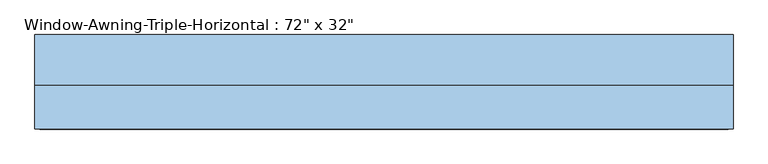
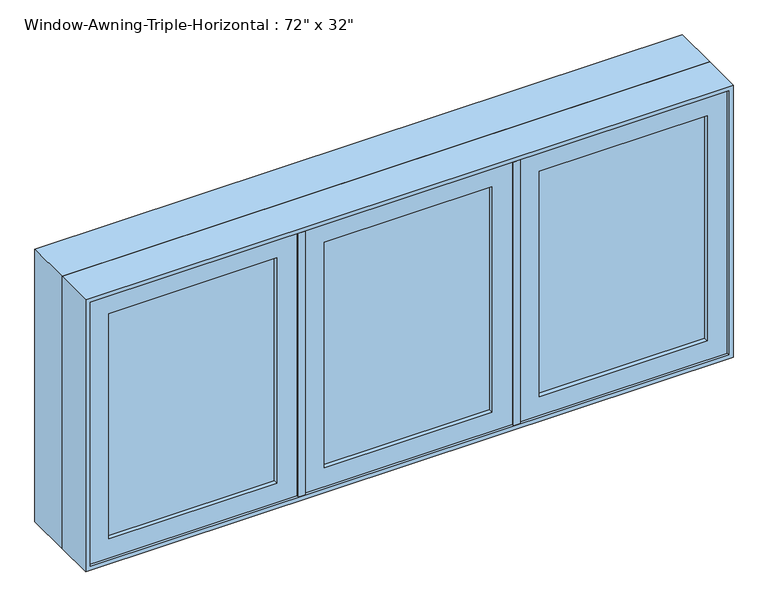
"""IFC4 building model written with IfcOpenShell, lengths in millimetres: window geometry."""

from ifc_helpers import new_model, si_unit, frame, origin, place, context, project, spatial, polyline, outline, extrude, faceted_brep, source, transform, mapped, element, save


def window_33d4544c(model_context):
    return source(origin(), model_context, "Body", "SolidModel", [
        faceted_brep([(882.65, -82.55, 1695.45), (-882.65, -82.55, 1695.45), (-882.65, -19.05, 1695.45), (882.65, -19.05, 1695.45), (901.7, -133.35, 1714.5), (-901.7, -133.35, 1714.5), (-901.7, -82.55, 1714.5), (901.7, -82.55, 1714.5), (914.4, -19.05, 1727.2), (-914.4, -19.05, 1727.2), (-914.4, -133.35, 1727.2), (914.4, -133.35, 1727.2), (-882.65, -82.55, 946.15), (-882.65, -19.05, 946.15), (-901.7, -133.35, 927.1), (-901.7, -82.55, 927.1), (-914.4, -19.05, 914.4), (-914.4, -133.35, 914.4), (882.65, -82.55, 946.15), (882.65, -19.05, 946.15), (901.7, -133.35, 927.1), (901.7, -82.55, 927.1), (914.4, -19.05, 914.4), (914.4, -133.35, 914.4)], [[[0, 1, 2, 3]], [[4, 5, 6, 7]], [[8, 9, 10, 11]], [[1, 12, 13, 2]], [[5, 14, 15, 6]], [[9, 16, 17, 10]], [[12, 18, 19, 13]], [[14, 20, 21, 15]], [[16, 22, 23, 17]], [[9, 8, 22, 16], [3, 2, 13, 19]], [[18, 0, 3, 19]], [[7, 6, 15, 21], [1, 0, 18, 12]], [[20, 4, 7, 21]], [[22, 8, 11, 23]], [[11, 10, 17, 23], [5, 4, 20, 14]]]),
        extrude(outline(polyline([(1727.2, -914.4), (914.4, -914.4), (914.4, 914.4), (1727.2, 914.4), (1727.2, -914.4)]), holes=[polyline([(1708.15, 895.35), (933.45, 895.35), (933.45, -895.35), (1708.15, -895.35), (1708.15, 895.35)])]), frame((0.0, -19.05, 0.0), z_axis=(0.0, 1.0, 0.0), x_axis=(0.0, 0.0, 1.0)), (0.0, 0.0, 1.0), 133.35),
        extrude(outline(polyline([(927.1, 313.2666667), (927.1, 901.7), (1714.5, 901.7), (1714.5, 313.2666667), (927.1, 313.2666667)]), holes=[polyline([(984.25, 844.55), (984.25, 370.4166667), (1657.35, 370.4166667), (1657.35, 844.55), (984.25, 844.55)])]), frame((0.0, -127.0, 0.0), z_axis=(0.0, 1.0, 0.0), x_axis=(0.0, 0.0, 1.0)), (0.0, 0.0, 1.0), 44.45),
        extrude(outline(polyline([(1714.5, -313.2666667), (1714.5, -901.7), (927.1, -901.7), (927.1, -313.2666667), (1714.5, -313.2666667)]), holes=[polyline([(1657.35, -844.55), (1657.35, -370.4166667), (984.25, -370.4166667), (984.25, -844.55), (1657.35, -844.55)])]), frame((0.0, -127.0, 0.0), z_axis=(0.0, 1.0, 0.0), x_axis=(0.0, 0.0, 1.0)), (0.0, 0.0, 1.0), 44.45),
        extrude(outline(polyline([(844.55, -114.3), (370.4166667, -114.3), (370.4166667, -107.95), (844.55, -107.95), (844.55, -114.3)])), frame((0.0, 0.0, 984.25), z_axis=(0.0, 0.0, 1.0), x_axis=(1.0, 0.0, 0.0)), (0.0, 0.0, 1.0), 673.1),
        extrude(outline(polyline([(370.4166667, -95.25), (844.55, -95.25), (844.55, -101.6), (370.4166667, -101.6), (370.4166667, -95.25)])), frame((0.0, 0.0, 984.25), z_axis=(0.0, 0.0, 1.0), x_axis=(1.0, 0.0, 0.0)), (0.0, 0.0, 1.0), 673.1),
        extrude(outline(polyline([(-370.4166667, -114.3), (-844.55, -114.3), (-844.55, -107.95), (-370.4166667, -107.95), (-370.4166667, -114.3)])), frame((0.0, 0.0, 984.25), z_axis=(0.0, 0.0, 1.0), x_axis=(1.0, 0.0, 0.0)), (0.0, 0.0, 1.0), 673.1),
        extrude(outline(polyline([(-844.55, -95.25), (-370.4166667, -95.25), (-370.4166667, -101.6), (-844.55, -101.6), (-844.55, -95.25)])), frame((0.0, 0.0, 984.25), z_axis=(0.0, 0.0, 1.0), x_axis=(1.0, 0.0, 0.0)), (0.0, 0.0, 1.0), 673.1),
        extrude(outline(polyline([(237.0666667, -114.3), (-237.0666667, -114.3), (-237.0666667, -107.95), (237.0666667, -107.95), (237.0666667, -114.3)])), frame((0.0, 0.0, 984.25), z_axis=(0.0, 0.0, 1.0), x_axis=(1.0, 0.0, 0.0)), (0.0, 0.0, 1.0), 673.1),
        extrude(outline(polyline([(-237.0666667, -95.25), (237.0666667, -95.25), (237.0666667, -101.6), (-237.0666667, -101.6), (-237.0666667, -95.25)])), frame((0.0, 0.0, 984.25), z_axis=(0.0, 0.0, 1.0), x_axis=(1.0, 0.0, 0.0)), (0.0, 0.0, 1.0), 673.1),
        extrude(outline(polyline([(927.1, -294.2166667), (927.1, 294.2166667), (1714.5, 294.2166667), (1714.5, -294.2166667), (927.1, -294.2166667)]), holes=[polyline([(984.25, 237.0666667), (984.25, -237.0666667), (1657.35, -237.0666667), (1657.35, 237.0666667), (984.25, 237.0666667)])]), frame((0.0, -127.0, 0.0), z_axis=(0.0, 1.0, 0.0), x_axis=(0.0, 0.0, 1.0)), (0.0, 0.0, 1.0), 44.45),
        faceted_brep([(294.2166667, -82.55, 1714.5), (294.2166667, -133.35, 1714.5), (313.2666667, -133.35, 1714.5), (313.2666667, -82.55, 1714.5), (333.7768005, -82.55, 1714.5), (333.7768005, -19.05, 1714.5), (273.7065328, -19.05, 1714.5), (273.7065328, -82.55, 1714.5), (294.2166667, -133.35, 927.1), (294.2166667, -104.775, 927.1), (313.2666667, -104.775, 927.1), (313.2666667, -133.35, 927.1), (273.7065328, -82.55, 1708.15), (294.2166667, -82.55, 1708.15), (294.2166667, -82.55, 1695.45), (273.7065328, -82.55, 1695.45), (273.7065328, -82.55, 946.15), (294.2166667, -82.55, 946.15), (273.7065328, -19.05, 1708.15), (273.7065328, -19.05, 1695.45), (273.7065328, -19.05, 946.15), (333.7768005, -19.05, 1708.15), (333.7768005, -19.05, 1695.45), (333.7768005, -19.05, 946.15), (333.7768005, -82.55, 1708.15), (333.7768005, -82.55, 1695.45), (333.7768005, -82.55, 946.15), (313.2666667, -82.55, 1708.15), (313.2666667, -82.55, 1695.45), (313.2666667, -82.55, 946.15), (313.2666667, -104.775, 946.15), (313.2666667, -104.775, 1695.45), (313.2666667, -104.775, 1708.15), (294.2166667, -104.775, 1708.15), (294.2166667, -104.775, 1695.45), (294.2166667, -104.775, 946.15)], [[[0, 1, 2, 3, 4, 5, 6, 7]], [[8, 9, 10, 11]], [[7, 12, 13, 0]], [[14, 15, 16, 17]], [[6, 18, 12, 7]], [[15, 19, 20, 16]], [[5, 21, 18, 6]], [[19, 22, 23, 20]], [[4, 24, 21, 5]], [[22, 25, 26, 23]], [[3, 27, 24, 4]], [[25, 28, 29, 26]], [[2, 11, 10, 30, 29, 28, 31, 32, 27, 3]], [[0, 13, 33, 34, 14, 17, 35, 9, 8, 1]], [[32, 31, 34, 33]], [[30, 10, 9, 35]], [[33, 13, 12, 18, 21, 24, 27, 32]], [[31, 28, 25, 22, 19, 15, 14, 34]], [[35, 17, 16, 20, 23, 26, 29, 30]], [[1, 8, 11, 2]]]),
        faceted_brep([(-313.2666667, -82.55, 1714.5), (-313.2666667, -133.35, 1714.5), (-294.2166667, -133.35, 1714.5), (-294.2166667, -82.55, 1714.5), (-273.7065328, -82.55, 1714.5), (-273.7065328, -19.05, 1714.5), (-333.7768005, -19.05, 1714.5), (-333.7768005, -82.55, 1714.5), (-313.2666667, -133.35, 927.1), (-313.2666667, -104.775, 927.1), (-294.2166667, -104.775, 927.1), (-294.2166667, -133.35, 927.1), (-333.7768005, -19.05, 1708.15), (-333.7768005, -82.55, 1708.15), (-333.7768005, -82.55, 1695.45), (-333.7768005, -19.05, 1695.45), (-333.7768005, -19.05, 946.15), (-333.7768005, -82.55, 946.15), (-273.7065328, -19.05, 1708.15), (-273.7065328, -19.05, 1695.45), (-273.7065328, -19.05, 946.15), (-273.7065328, -82.55, 1708.15), (-273.7065328, -82.55, 1695.45), (-273.7065328, -82.55, 946.15), (-294.2166667, -104.775, 946.15), (-294.2166667, -82.55, 946.15), (-294.2166667, -82.55, 1695.45), (-294.2166667, -104.775, 1695.45), (-294.2166667, -104.775, 1708.15), (-294.2166667, -82.55, 1708.15), (-313.2666667, -82.55, 1708.15), (-313.2666667, -104.775, 1708.15), (-313.2666667, -104.775, 1695.45), (-313.2666667, -82.55, 1695.45), (-313.2666667, -82.55, 946.15), (-313.2666667, -104.775, 946.15)], [[[0, 1, 2, 3, 4, 5, 6, 7]], [[8, 9, 10, 11]], [[6, 12, 13, 7]], [[14, 15, 16, 17]], [[5, 18, 12, 6]], [[15, 19, 20, 16]], [[4, 21, 18, 5]], [[19, 22, 23, 20]], [[2, 11, 10, 24, 25, 26, 27, 28, 29, 3]], [[0, 30, 31, 32, 33, 34, 35, 9, 8, 1]], [[28, 27, 32, 31]], [[24, 10, 9, 35]], [[31, 30, 13, 12, 18, 21, 29, 28]], [[27, 26, 22, 19, 15, 14, 33, 32]], [[35, 34, 17, 16, 20, 23, 25, 24]], [[7, 13, 30, 0]], [[17, 34, 33, 14]], [[3, 29, 21, 4]], [[25, 23, 22, 26]], [[1, 8, 11, 2]]]),
    ])


if __name__ == "__main__":
    model = new_model("IFC4")
    model_context = context("Model", 3, world=origin())
    ifc_project = project(units=[si_unit("LENGTHUNIT", "METRE", prefix="MILLI")], contexts=[model_context])
    site = spatial("IfcSite", under=ifc_project)
    building = spatial("IfcBuilding", under=site)
    placement = place(None, origin())
    window_shape = window_33d4544c(model_context)
    element("IfcWindow", 1, ObjectType="Window-Awning-Triple-Horizontal : 72\" x 32\"", at=placement, inside=building, context=model_context, shape_type="MappedRepresentation", body=[
        mapped(window_shape, transform((0.0, 0.0, 0.0), x_axis=(1.0, 0.0, 0.0), y_axis=(0.0, 1.0, 0.0), z_axis=(0.0, 0.0, 1.0))),
    ])
    save(model, "model.ifc")

# Revit data of these elements
# Type "Window-Awning-Triple-Horizontal : 72\" x 32\""
#   Type Mark = "31"
#   Fire Rating = "0.5h"
#   Assembly Code = "B2020100"
#   Analytic Construction = "Double glazing - domestic"
#   Window Inset [instance default] = 0 ft
#   Wall Thickness [instance default] = 0.5 ft
#   Muntin Width = 1.555556 ft
#   Visual Light Transmittance = 0.81
#   Thermal Resistance (R) = 1.8146 (h·ft²·°F)/BTU
#   Solar Heat Gain Coefficient = 0.76
#   One Third Width = 2 ft
#   Sash Width = 1.930556 ft
#   Rough Width = 6.041667 ft
#   Rough Height = 2.708333 ft
#   Interior Wall Closure [instance default] = 0.1875 ft
#   Height = 2.666667 ft
#   Heat Transfer Coefficient (U) = 0.5511 BTU/(h·ft²·°F)
#   Muntin Height = 2.208333 ft
#   Frame Extension [instance default] = 0.020833 ft
#   Exterior Wall Closure [instance default] = 0.104167 ft
#   Extension Jamb [instance default] = 0.1875 ft
#   Default Sill Height = 3 ft
#   Width = 6 ft
#   Middle Muntin Visibility = yes
#   Side Muntin Visibility = yes
#   Interior Trim Visibility [instance default] = yes
#   Exterior Trim Visibility [instance default] = yes
#   Extension Jamb Visibility [instance default] = yes
#   Muntin Pattern = Muntin Pattern_2x2 : Muntin Pattern_2x2
#   Interior Trim Material = Wood - Stained
#   Interior Trim = Trim-Window-Interior-Flat : Picture Frame
#   Interior Frame Material = Wood - Stained
#   Glass Panel Material = Glass
#   Exterior Trim Material = Clad - White
#   Exterior Trim = Trim-Window-Exterior-Flat : with Sill
#   Exterior Frame Material = Clad - White
#   Wall Closure = (empty or 0)
# Element 1 (IfcWindow, "Window-Awning-Triple-Horizontal : 72\" x 32\"")
#   Wall Thickness = 0.75 ft
#   Extension Jamb = 0.4375 ft
#   Materials on its faces: "Wood - Stained", "Glass", "Clad - White"
# Materials
#   "Wood - Stained": class "Wood", colour RGB 224 178 126, transparency 0, Cost = 0
#   "Glass": class "Glass", colour RGB 0 128 192, transparency 0.75, Description = "Soda Lime Glass", Cost = 0
#   "Clad - White": class "Wood", colour RGB 242 242 238, transparency 0, Cost = 0
